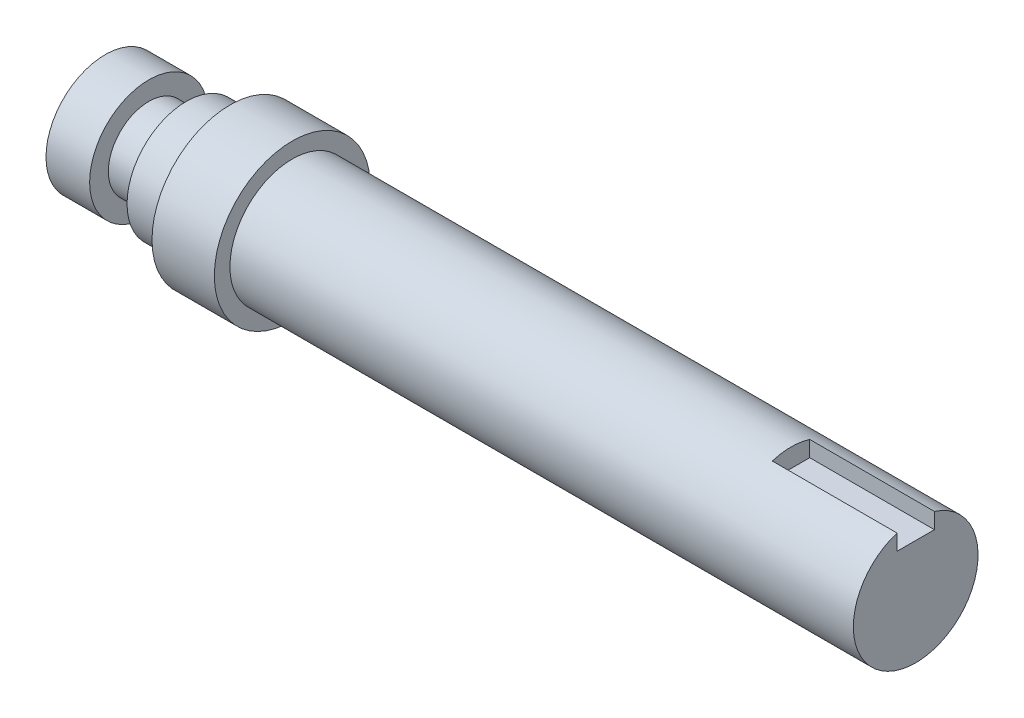
from build123d import *

# Parameters (mm, degrees)
KEYWAY_SKETCH_W  = 20
KEYWAY_SKETCH_H  = 5
KEYWAY_CUT_DEPTH = 3


with BuildPart() as part:
    # Shaft Profile Sketch → Stepped Shaft Body (revolve)
    with BuildSketch(Plane.XY, mode=Mode.PRIVATE) as stepped_shaft_body_sk:
        Polygon((0, 0), (0, 9.5), (7, 9.5), (7, 6.5), (13, 6.5), (13, 9.5), (20, 9.5), (20, 12.5), (30, 12.5), (30, 10), (130, 10), (130, 0), align=None)
    revolve(stepped_shaft_body_sk.sketch.rotate(Axis((0, 0, 0), (1, 0, 0)), 90), axis=Axis((0, 0, 0), (1, 0, 0)))

    # Keyway Sketch → Keyway Cut (cut, symmetric)
    with BuildSketch(Plane.XY):
        with Locations((120, 9.5)):
            Rectangle(KEYWAY_SKETCH_W, KEYWAY_SKETCH_H)
    extrude(amount=KEYWAY_CUT_DEPTH, both=True, mode=Mode.SUBTRACT)


solid = part.part
